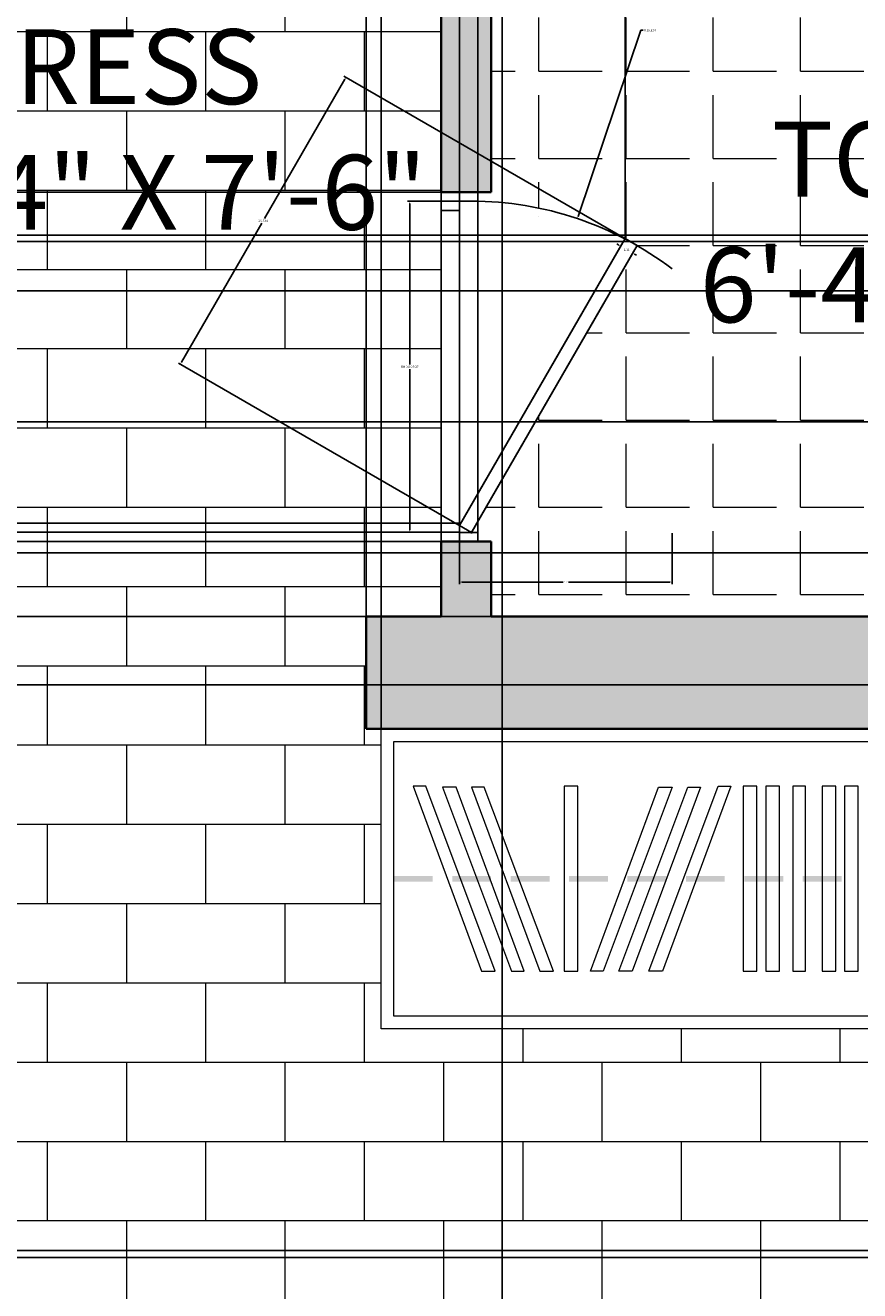
# Model space of a CAD drawing. Units: inches. Extents: x 6 to 575, y 34 to 566.
# Tile 7 of 21: x 84 to 151, y 387 to 488. Entities that reach past the tile are written whole.
import ezdxf

# ---------------------------------------------------------------- set-up
doc = ezdxf.new("R2010")
doc.units = ezdxf.units.IN
for name, color, linetype, lineweight in [('A-ANNO-DIMS', 2, 'Continuous', 18), ('A-AREA-IDEN', 6, 'Continuous', 20), ('A-DOOR-THRS', 8, 'Continuous', 13), ('A-FLOR-CASE', 2, 'Continuous', 18), ('A-FLOR-PATT', 252, 'Continuous', 9), ('A-WALL-PATT', 251, 'Continuous', 9), ('DOORS', 3, 'Continuous', 25), ('WALLS', 7, 'Continuous', 35)]:
    doc.layers.add(name, color=color, linetype=linetype, lineweight=lineweight)
doc.styles.add('PDF Arial Narrow', font='txt')
doc.styles.get("Standard").update_dxf_attribs({"font": 'arial.ttf'})
doc.dimstyles.get("Standard").update_dxf_attribs({"dimtxt": 0.18, "dimasz": 0.18, "dimexe": 0.18, "dimexo": 0.0625, "dimgap": 0.09, "dimtad": 0, "dimtih": 1, "dimtoh": 1, "dimdec": 4, "dimzin": 0, "dimdsep": 46, "dimtxsty": 'Standard', "dimcen": 0.09, "dimadec": 0, "dimazin": 0, "dimtfac": 1, "dimtdec": 4, "dimtofl": 0, "dimtmove": 0, "dimatfit": 3, "dimfxl": 1, "dimtolj": 1, "dimtzin": 0, "dimarcsym": 0})

# ---------------------------------------------------------------- blocks, each defined once
blk = doc.blocks.new('Door - Right Hung 36 in.')
blk.add_lwpolyline([(-0.75, -1.3), (0, 0), (-31.18, 18), (-31.93, 16.7)], close=True)
blk.add_arc((0, 0), 36, 142.6899, 180)
blk = doc.blocks.new('*D17')
at = {"layer": 'A-ANNO-DIMS', "color": 0, "lineweight": -2, "transparency": 16777216}
for p, q in [((119.07, 474.07), (114.97, 474.07)), ((115.15, 473.89), (115.15, 460.99)), ((115.15, 447.72), (115.15, 460.62)), ((119.07, 447.54), (114.97, 447.54))]:
    blk.add_line(p, q, dxfattribs=at)
at = {"layer": 'A-ANNO-DIMS', "color": 0, "transparency": 16777216}
for points in [[(115.12, 473.89), (115.18, 473.89), (115.15, 474.07)], [(115.12, 447.72), (115.18, 447.72), (115.15, 447.54)]]:
    blk.add_solid(points, dxfattribs=at)
at = {"layer": 'Defpoints', "color": 0, "transparency": 16777216}
for p in [(119.13, 474.07), (115.15, 447.54), (119.13, 447.54)]:
    blk.add_point(p, dxfattribs=at)
at = {"layer": 'A-ANNO-DIMS', "color": 0, "transparency": 16777216, "insert": (115.15, 460.8), "char_height": 0.18, "attachment_point": 5}
blk.add_mtext('\\A1;RH DOOR 27', dxfattribs=at)
blk = doc.blocks.new('*D18')
at = {"layer": 'A-ANNO-DIMS', "color": 0, "lineweight": -2, "transparency": 16777216}
for p, q in [((119.13, 447.48), (119.13, 443.38)), ((136.17, 447.48), (136.17, 443.38)), ((119.31, 443.56), (127.44, 443.56)), ((135.99, 443.56), (127.86, 443.56))]:
    blk.add_line(p, q, dxfattribs=at)
at = {"layer": 'A-ANNO-DIMS', "color": 0, "transparency": 16777216}
for points in [[(119.31, 443.59), (119.31, 443.53), (119.13, 443.56)], [(135.99, 443.59), (135.99, 443.53), (136.17, 443.56)]]:
    blk.add_solid(points, dxfattribs=at)
at = {"layer": 'Defpoints', "color": 0, "transparency": 16777216}
for p in [(119.13, 447.54), (136.17, 447.54), (136.17, 443.56)]:
    blk.add_point(p, dxfattribs=at)
at = {"layer": 'A-ANNO-DIMS', "color": 0, "transparency": 16777216, "insert": (127.65, 443.56), "char_height": 0.18, "attachment_point": 5}
blk.add_mtext('\\A1;17', dxfattribs=at)
blk = doc.blocks.new('*D30')
at = {"layer": 'A-ANNO-DIMS', "color": 0, "lineweight": -2, "transparency": 16777216}
for p, q in [((32.6, 539.8), (6.65, 539.8)), ((6.83, 539.62), (6.83, 299.97)), ((6.83, 59.95), (6.83, 299.61)), ((197.62, 59.77), (6.65, 59.77))]:
    blk.add_line(p, q, dxfattribs=at)
at = {"layer": 'A-ANNO-DIMS', "color": 0, "transparency": 16777216}
for points in [[(6.8, 539.62), (6.86, 539.62), (6.83, 539.8)], [(6.8, 59.95), (6.86, 59.95), (6.83, 59.77)]]:
    blk.add_solid(points, dxfattribs=at)
at = {"layer": 'Defpoints', "color": 0, "transparency": 16777216}
for p in [(32.66, 539.8), (6.83, 59.77), (197.69, 59.77)]:
    blk.add_point(p, dxfattribs=at)
at = {"layer": 'A-ANNO-DIMS', "color": 0, "transparency": 16777216, "insert": (6.83, 299.79), "char_height": 0.18, "attachment_point": 5}
blk.add_mtext('\\A1;480', dxfattribs=at)
blk = doc.blocks.new('*D52')
at = {"layer": 'A-ANNO-DIMS', "color": 0, "lineweight": -2, "transparency": 16777216}
for p, q in [((437.62, 471.35), (6.65, 471.35)), ((6.83, 471.17), (6.83, 453.51)), ((6.83, 435.49), (6.83, 453.15)), ((437.62, 435.31), (6.65, 435.31))]:
    blk.add_line(p, q, dxfattribs=at)
at = {"layer": 'A-ANNO-DIMS', "color": 0, "transparency": 16777216}
for points in [[(6.8, 471.17), (6.86, 471.17), (6.83, 471.35)], [(6.8, 435.49), (6.86, 435.49), (6.83, 435.31)]]:
    blk.add_solid(points, dxfattribs=at)
at = {"layer": 'Defpoints', "color": 0, "transparency": 16777216}
for p in [(6.83, 471.35), (437.69, 471.35), (437.69, 435.31)]:
    blk.add_point(p, dxfattribs=at)
at = {"layer": 'A-ANNO-DIMS', "color": 0, "transparency": 16777216, "insert": (6.83, 453.33), "char_height": 0.18, "attachment_point": 5}
blk.add_mtext('\\A1;36.045', dxfattribs=at)
blk = doc.blocks.new('*D55')
at = {"layer": 'A-ANNO-DIMS', "color": 0, "lineweight": -2, "transparency": 16777216}
for p, q in [((41.66, 286.13), (41.66, 565.81)), ((122.56, 286.13), (122.56, 565.81)), ((41.84, 565.63), (81.79, 565.63)), ((122.38, 565.63), (82.44, 565.63))]:
    blk.add_line(p, q, dxfattribs=at)
at = {"layer": 'A-ANNO-DIMS', "color": 0, "transparency": 16777216}
for points in [[(41.84, 565.66), (41.84, 565.6), (41.66, 565.63)], [(122.38, 565.66), (122.38, 565.6), (122.56, 565.63)]]:
    blk.add_solid(points, dxfattribs=at)
at = {"layer": 'Defpoints', "color": 0, "transparency": 16777216}
for p in [(122.56, 565.63), (41.66, 286.06), (122.56, 286.06)]:
    blk.add_point(p, dxfattribs=at)
at = {"layer": 'A-ANNO-DIMS', "color": 0, "transparency": 16777216, "insert": (82.11, 565.63), "char_height": 0.18, "attachment_point": 5}
blk.add_mtext('\\A1;80.9', dxfattribs=at)
blk = doc.blocks.new('*D67')
at = {"layer": 'A-ANNO-DIMS', "color": 0, "lineweight": -2, "transparency": 16777216}
for p, q in [((82.89, 440.86), (82.89, 565.81)), ((111.66, 440.86), (111.66, 565.81)), ((83.07, 565.63), (96.81, 565.63)), ((111.48, 565.63), (97.74, 565.63))]:
    blk.add_line(p, q, dxfattribs=at)
at = {"layer": 'A-ANNO-DIMS', "color": 0, "transparency": 16777216}
for points in [[(83.07, 565.66), (83.07, 565.6), (82.89, 565.63)], [(111.48, 565.66), (111.48, 565.6), (111.66, 565.63)]]:
    blk.add_solid(points, dxfattribs=at)
at = {"layer": 'Defpoints', "color": 0, "transparency": 16777216}
for p in [(111.66, 565.63), (82.89, 440.8), (111.66, 440.8)]:
    blk.add_point(p, dxfattribs=at)
at = {"layer": 'A-ANNO-DIMS', "color": 0, "transparency": 16777216, "insert": (97.28, 565.63), "char_height": 0.18, "attachment_point": 5}
blk.add_mtext('\\A1;28.767', dxfattribs=at)
blk = doc.blocks.new('*D109')
at = {"layer": 'A-ANNO-DIMS', "color": 0, "lineweight": -2, "transparency": 16777216}
for p, q in [((112.85, 431.86), (112.85, 565.81)), ((197.66, 431.86), (197.66, 565.81)), ((113.03, 565.63), (154.93, 565.63)), ((197.48, 565.63), (155.58, 565.63))]:
    blk.add_line(p, q, dxfattribs=at)
at = {"layer": 'A-ANNO-DIMS', "color": 0, "transparency": 16777216}
for points in [[(113.03, 565.66), (113.03, 565.6), (112.85, 565.63)], [(197.48, 565.66), (197.48, 565.6), (197.66, 565.63)]]:
    blk.add_solid(points, dxfattribs=at)
at = {"layer": 'Defpoints', "color": 0, "transparency": 16777216}
for p in [(197.66, 565.63), (112.85, 431.8), (197.66, 431.8)]:
    blk.add_point(p, dxfattribs=at)
at = {"layer": 'A-ANNO-DIMS', "color": 0, "transparency": 16777216, "insert": (155.25, 565.63), "char_height": 0.18, "attachment_point": 5}
blk.add_mtext('\\A1;84.8', dxfattribs=at)
blk = doc.blocks.new('*D132')
at = {"layer": 'A-ANNO-DIMS', "color": 0, "lineweight": -2, "transparency": 16777216}
for p, q in [((288.54, 390), (6.65, 390)), ((6.83, 389.82), (6.83, 366.19)), ((6.83, 342.19), (6.83, 365.82)), ((288.54, 342.01), (6.65, 342.01))]:
    blk.add_line(p, q, dxfattribs=at)
at = {"layer": 'A-ANNO-DIMS', "color": 0, "transparency": 16777216}
for points in [[(6.8, 389.82), (6.86, 389.82), (6.83, 390)], [(6.8, 342.19), (6.86, 342.19), (6.83, 342.01)]]:
    blk.add_solid(points, dxfattribs=at)
at = {"layer": 'Defpoints', "color": 0, "transparency": 16777216}
for p in [(6.83, 390), (288.6, 390), (288.6, 342.01)]:
    blk.add_point(p, dxfattribs=at)
at = {"layer": 'A-ANNO-DIMS', "color": 0, "transparency": 16777216, "insert": (6.83, 366), "char_height": 0.18, "attachment_point": 5}
blk.add_mtext('\\A1;47.98', dxfattribs=at)
blk = doc.blocks.new('*D136')
at = {"layer": 'A-ANNO-DIMS', "color": 0, "lineweight": -2, "transparency": 16777216}
for p, q in [((206.62, 389.45), (6.65, 389.45)), ((6.83, 389.27), (6.83, 350.19)), ((6.83, 310.75), (6.83, 349.83)), ((206.62, 310.57), (6.65, 310.57))]:
    blk.add_line(p, q, dxfattribs=at)
at = {"layer": 'A-ANNO-DIMS', "color": 0, "transparency": 16777216}
for points in [[(6.8, 389.27), (6.86, 389.27), (6.83, 389.45)], [(6.8, 310.75), (6.86, 310.75), (6.83, 310.57)]]:
    blk.add_solid(points, dxfattribs=at)
at = {"layer": 'Defpoints', "color": 0, "transparency": 16777216}
for p in [(6.83, 389.45), (206.68, 389.45), (206.68, 310.57)]:
    blk.add_point(p, dxfattribs=at)
at = {"layer": 'A-ANNO-DIMS', "color": 0, "transparency": 16777216, "insert": (6.83, 350.01), "char_height": 0.18, "attachment_point": 5}
blk.add_mtext('\\A1;78.88', dxfattribs=at)
blk = doc.blocks.new('*D186')
at = {"layer": 'A-ANNO-DIMS', "color": 0, "lineweight": -2, "transparency": 16777216}
for p, q in [((197.6, 470.84), (6.65, 470.84)), ((6.83, 470.66), (6.83, 456)), ((6.83, 440.98), (6.83, 455.64)), ((176.61, 440.8), (6.65, 440.8))]:
    blk.add_line(p, q, dxfattribs=at)
at = {"layer": 'A-ANNO-DIMS', "color": 0, "transparency": 16777216}
for points in [[(6.8, 470.66), (6.86, 470.66), (6.83, 470.84)], [(6.8, 440.98), (6.86, 440.98), (6.83, 440.8)]]:
    blk.add_solid(points, dxfattribs=at)
at = {"layer": 'Defpoints', "color": 0, "transparency": 16777216}
for p in [(6.83, 470.84), (197.66, 470.84), (176.67, 440.8)]:
    blk.add_point(p, dxfattribs=at)
at = {"layer": 'A-ANNO-DIMS', "color": 0, "transparency": 16777216, "insert": (6.83, 455.82), "char_height": 0.18, "attachment_point": 5}
blk.add_mtext('\\A1;30.04', dxfattribs=at)
blk = doc.blocks.new('*D188')
at = {"layer": 'A-ANNO-DIMS', "color": 0, "lineweight": -2, "transparency": 16777216}
for p, q in [((187.14, 466.88), (6.65, 466.88)), ((6.83, 466.7), (6.83, 456.56)), ((6.83, 446.07), (6.83, 456.2)), ((187.02, 445.89), (6.65, 445.89))]:
    blk.add_line(p, q, dxfattribs=at)
at = {"layer": 'A-ANNO-DIMS', "color": 0, "transparency": 16777216}
for points in [[(6.8, 466.7), (6.86, 466.7), (6.83, 466.88)], [(6.8, 446.07), (6.86, 446.07), (6.83, 445.89)]]:
    blk.add_solid(points, dxfattribs=at)
at = {"layer": 'Defpoints', "color": 0, "transparency": 16777216}
for p in [(6.83, 466.88), (187.2, 466.88), (187.08, 445.89)]:
    blk.add_point(p, dxfattribs=at)
at = {"layer": 'A-ANNO-DIMS', "color": 0, "transparency": 16777216, "insert": (6.83, 456.38), "char_height": 0.18, "attachment_point": 5}
blk.add_mtext('\\A1;20.987', dxfattribs=at)
blk = doc.blocks.new('*D189')
at = {"layer": 'A-ANNO-DIMS', "color": 0, "lineweight": -2, "transparency": 16777216}
for p, q in [((187.08, 456.38), (6.65, 456.38)), ((6.83, 456.2), (6.83, 448.77)), ((6.83, 440.98), (6.83, 448.41)), ((197.6, 440.8), (6.65, 440.8))]:
    blk.add_line(p, q, dxfattribs=at)
at = {"layer": 'A-ANNO-DIMS', "color": 0, "transparency": 16777216}
for points in [[(6.8, 456.2), (6.86, 456.2), (6.83, 456.38)], [(6.8, 440.98), (6.86, 440.98), (6.83, 440.8)]]:
    blk.add_solid(points, dxfattribs=at)
at = {"layer": 'Defpoints', "color": 0, "transparency": 16777216}
for p in [(6.83, 456.38), (187.14, 456.38), (197.66, 440.8)]:
    blk.add_point(p, dxfattribs=at)
at = {"layer": 'A-ANNO-DIMS', "color": 0, "transparency": 16777216, "insert": (6.83, 448.59), "char_height": 0.18, "attachment_point": 5}
blk.add_mtext('\\A1;15.582', dxfattribs=at)
blk = doc.blocks.new('*D197')
at = {"layer": 'A-ANNO-DIMS', "color": 0, "lineweight": -2, "transparency": 16777216}
for p, q in [((117.6, 446.8), (6.65, 446.8)), ((6.83, 446.62), (6.83, 443.98)), ((6.83, 440.98), (6.83, 443.62)), ((117.6, 440.8), (6.65, 440.8))]:
    blk.add_line(p, q, dxfattribs=at)
at = {"layer": 'A-ANNO-DIMS', "color": 0, "transparency": 16777216}
for points in [[(6.8, 446.62), (6.86, 446.62), (6.83, 446.8)], [(6.8, 440.98), (6.86, 440.98), (6.83, 440.8)]]:
    blk.add_solid(points, dxfattribs=at)
at = {"layer": 'Defpoints', "color": 0, "transparency": 16777216}
for p in [(6.83, 446.8), (117.66, 446.8), (117.66, 440.8)]:
    blk.add_point(p, dxfattribs=at)
at = {"layer": 'A-ANNO-DIMS', "color": 0, "transparency": 16777216, "insert": (6.83, 443.8), "char_height": 0.18, "attachment_point": 5}
blk.add_mtext('\\A1;6', dxfattribs=at)
blk = doc.blocks.new('*D198')
at = {"layer": 'A-ANNO-DIMS', "color": 0, "lineweight": -2, "transparency": 16777216}
for p, q in [((117.6, 474.8), (6.65, 474.8)), ((6.83, 474.62), (6.83, 460.98)), ((6.83, 446.98), (6.83, 460.62)), ((117.6, 446.8), (6.65, 446.8))]:
    blk.add_line(p, q, dxfattribs=at)
at = {"layer": 'A-ANNO-DIMS', "color": 0, "transparency": 16777216}
for points in [[(6.8, 474.62), (6.86, 474.62), (6.83, 474.8)], [(6.8, 446.98), (6.86, 446.98), (6.83, 446.8)]]:
    blk.add_solid(points, dxfattribs=at)
at = {"layer": 'Defpoints', "color": 0, "transparency": 16777216}
for p in [(6.83, 474.8), (117.66, 474.8), (117.66, 446.8)]:
    blk.add_point(p, dxfattribs=at)
at = {"layer": 'A-ANNO-DIMS', "color": 0, "transparency": 16777216, "insert": (6.83, 460.8), "char_height": 0.18, "attachment_point": 5}
blk.add_mtext('\\A1;28', dxfattribs=at)
blk = doc.blocks.new('*D199')
at = {"layer": 'A-ANNO-DIMS', "color": 0, "lineweight": -2, "transparency": 16777216}
for p, q in [((109.94, 483.83), (103.5, 472.68)), ((132.35, 471.1), (109.87, 484.07)), ((96.85, 461.16), (103.29, 472.31)), ((119.08, 448.12), (96.61, 461.1))]:
    blk.add_line(p, q, dxfattribs=at)
at = {"layer": 'A-ANNO-DIMS', "color": 0, "transparency": 16777216}
for points in [[(109.91, 483.84), (109.97, 483.81), (110.03, 483.98)], [(96.83, 461.18), (96.88, 461.15), (96.76, 461.01)]]:
    blk.add_solid(points, dxfattribs=at)
at = {"layer": 'Defpoints', "color": 0, "transparency": 16777216}
for p in [(110.03, 483.98), (132.4, 471.07), (119.13, 448.09)]:
    blk.add_point(p, dxfattribs=at)
at = {"layer": 'A-ANNO-DIMS', "color": 0, "transparency": 16777216, "insert": (103.4, 472.5), "char_height": 0.18, "attachment_point": 5}
blk.add_mtext('\\A1;26.534', dxfattribs=at)
blk = doc.blocks.new('*D200')
at = {"layer": 'A-ANNO-DIMS', "color": 0, "lineweight": -2, "transparency": 16777216}
for p, q in [((119.13, 448.15), (119.13, 565.81)), ((132.4, 471.13), (132.4, 565.81)), ((119.31, 565.63), (125.31, 565.63)), ((132.22, 565.63), (126.22, 565.63))]:
    blk.add_line(p, q, dxfattribs=at)
at = {"layer": 'A-ANNO-DIMS', "color": 0, "transparency": 16777216}
for points in [[(119.31, 565.66), (119.31, 565.6), (119.13, 565.63)], [(132.22, 565.66), (132.22, 565.6), (132.4, 565.63)]]:
    blk.add_solid(points, dxfattribs=at)
at = {"layer": 'Defpoints', "color": 0, "transparency": 16777216}
for p in [(132.4, 565.63), (132.4, 471.07), (119.13, 448.09)]:
    blk.add_point(p, dxfattribs=at)
at = {"layer": 'A-ANNO-DIMS', "color": 0, "transparency": 16777216, "insert": (125.77, 565.63), "char_height": 0.18, "attachment_point": 5}
blk.add_mtext('\\A1;13.267', dxfattribs=at)
blk = doc.blocks.new('*D201')
at = {"layer": 'A-ANNO-DIMS', "color": 0, "lineweight": -2, "transparency": 16777216}
for p, q in [((119.16, 448.14), (132.14, 470.62)), ((131.89, 470.55), (131.74, 470.64)), ((120.12, 447.59), (133.1, 470.06)), ((133.16, 469.82), (133.32, 469.73))]:
    blk.add_line(p, q, dxfattribs=at)
at = {"layer": 'A-ANNO-DIMS', "color": 0, "transparency": 16777216}
for points in [[(131.91, 470.58), (131.88, 470.52), (132.05, 470.46)], [(133.18, 469.84), (133.15, 469.79), (133.01, 469.91)]]:
    blk.add_solid(points, dxfattribs=at)
at = {"layer": 'Defpoints', "color": 0, "transparency": 16777216}
for p in [(133.01, 469.91), (119.13, 448.09), (120.09, 447.54)]:
    blk.add_point(p, dxfattribs=at)
at = {"layer": 'A-ANNO-DIMS', "color": 0, "transparency": 16777216, "insert": (132.53, 470.18), "char_height": 0.18, "attachment_point": 5}
blk.add_mtext('\\A1;1.11', dxfattribs=at)
blk = doc.blocks.new('*D202')
at = {"layer": 'A-ANNO-DIMS', "color": 0, "lineweight": -2, "transparency": 16777216}
for p, q in [((117.66, 446.86), (117.66, 565.81)), ((120.61, 446.86), (120.61, 565.81)), ((117.84, 565.63), (118.74, 565.63)), ((120.43, 565.63), (119.53, 565.63))]:
    blk.add_line(p, q, dxfattribs=at)
at = {"layer": 'A-ANNO-DIMS', "color": 0, "transparency": 16777216}
for points in [[(117.84, 565.66), (117.84, 565.6), (117.66, 565.63)], [(120.43, 565.66), (120.43, 565.6), (120.61, 565.63)]]:
    blk.add_solid(points, dxfattribs=at)
at = {"layer": 'Defpoints', "color": 0, "transparency": 16777216}
for p in [(120.61, 565.63), (117.66, 446.8), (120.61, 446.8)]:
    blk.add_point(p, dxfattribs=at)
at = {"layer": 'A-ANNO-DIMS', "color": 0, "transparency": 16777216, "insert": (119.13, 565.63), "char_height": 0.18, "attachment_point": 5}
blk.add_mtext('\\A1;2.948', dxfattribs=at)
blk = doc.blocks.new('*D203')
at = {"layer": 'A-ANNO-DIMS', "color": 0, "lineweight": -2, "transparency": 16777216}
for p, q in [((117.6, 448.28), (6.65, 448.28)), ((6.83, 448.1), (6.83, 447.72)), ((6.83, 446.98), (6.83, 447.36)), ((117.6, 446.8), (6.65, 446.8))]:
    blk.add_line(p, q, dxfattribs=at)
at = {"layer": 'A-ANNO-DIMS', "color": 0, "transparency": 16777216}
for points in [[(6.8, 448.1), (6.86, 448.1), (6.83, 448.28)], [(6.8, 446.98), (6.86, 446.98), (6.83, 446.8)]]:
    blk.add_solid(points, dxfattribs=at)
at = {"layer": 'Defpoints', "color": 0, "transparency": 16777216}
for p in [(6.83, 448.28), (117.66, 448.28), (117.66, 446.8)]:
    blk.add_point(p, dxfattribs=at)
at = {"layer": 'A-ANNO-DIMS', "color": 0, "transparency": 16777216, "insert": (6.83, 447.54), "char_height": 0.18, "attachment_point": 5}
blk.add_mtext('\\A1;1.474', dxfattribs=at)
blk = doc.blocks.new('*D204')
at = {"layer": 'A-ANNO-DIMS', "color": 0, "lineweight": -2, "transparency": 16777216}
for p, q in [((119.07, 448.28), (6.65, 448.28)), ((6.83, 448.1), (6.83, 447.72)), ((119.07, 447.54), (6.65, 447.54)), ((6.83, 447.36), (6.65, 447.36)), ((6.83, 447.54), (6.83, 447.36))]:
    blk.add_line(p, q, dxfattribs=at)
at = {"layer": 'A-ANNO-DIMS', "color": 0, "transparency": 16777216}
for points in [[(6.8, 448.1), (6.86, 448.1), (6.83, 448.28)], [(6.8, 447.72), (6.86, 447.72), (6.83, 447.54)]]:
    blk.add_solid(points, dxfattribs=at)
at = {"layer": 'Defpoints', "color": 0, "transparency": 16777216}
for p in [(119.13, 448.28), (6.83, 447.54), (119.13, 447.54)]:
    blk.add_point(p, dxfattribs=at)
at = {"layer": 'A-ANNO-DIMS', "color": 0, "transparency": 16777216, "insert": (6.25, 447.36), "char_height": 0.18, "attachment_point": 5}
blk.add_mtext('\\A1;0.737', dxfattribs=at)
blk = doc.blocks.new('*D205')
at = {"layer": 'A-ANNO-DIMS', "color": 0, "lineweight": -2, "transparency": 16777216}
for p, q in [((119.13, 447.6), (119.13, 565.81)), ((120.61, 447.6), (120.61, 565.81)), ((119.31, 565.63), (119.48, 565.63)), ((120.43, 565.63), (120.25, 565.63))]:
    blk.add_line(p, q, dxfattribs=at)
at = {"layer": 'A-ANNO-DIMS', "color": 0, "transparency": 16777216}
for points in [[(119.31, 565.66), (119.31, 565.6), (119.13, 565.63)], [(120.43, 565.66), (120.43, 565.6), (120.61, 565.63)]]:
    blk.add_solid(points, dxfattribs=at)
at = {"layer": 'Defpoints', "color": 0, "transparency": 16777216}
for p in [(120.61, 565.63), (119.13, 447.54), (120.61, 447.54)]:
    blk.add_point(p, dxfattribs=at)
at = {"layer": 'A-ANNO-DIMS', "color": 0, "transparency": 16777216, "insert": (119.87, 565.63), "char_height": 0.18, "attachment_point": 5}
blk.add_mtext('\\A1;1.474', dxfattribs=at)
blk = doc.blocks.new('*D229')
at = {"layer": 'A-ANNO-DIMS', "color": 0, "lineweight": -2, "transparency": 16777216}
for p, q in [((133.67, 487.76), (128.63, 472.85)), ((133.85, 487.76), (133.67, 487.76)), ((120, 447.54), (120.18, 447.54)), ((120.09, 447.45), (120.09, 447.63))]:
    blk.add_line(p, q, dxfattribs=at)
at = {"layer": 'A-ANNO-DIMS', "color": 0, "transparency": 16777216}
blk.add_solid([(128.61, 472.86), (128.66, 472.84), (128.58, 472.68)], dxfattribs=at)
at = {"layer": 'Defpoints', "color": 0, "transparency": 16777216}
for p in [(128.58, 472.68), (120.09, 447.54)]:
    blk.add_point(p, dxfattribs=at)
at = {"layer": 'A-ANNO-DIMS', "color": 0, "transparency": 16777216, "insert": (134.4, 487.76), "char_height": 0.18, "attachment_point": 5}
blk.add_mtext('\\A1;R26.534', dxfattribs=at)

msp = doc.modelspace()

# ---------------------------------------------------------------- hatches: boundary and pattern name
at = {"layer": 'A-FLOR-PATT'}
h = msp.add_hatch(dxfattribs=at)
h.set_pattern_fill('ANGLE', color=256)
h.set_pattern_definition([(0, (-98.035, 170.1465), (0, 6.985), [5.08, -1.905]), (90, (-98.035, 170.1465), (-6.985, 4e-16), [5.08, -1.905])])
edge = h.paths.add_edge_path()
edge.add_line((191.6511, 494.1664), (190.4028, 493.9036))
edge.add_line((190.4028, 493.9036), (189.6226, 493.6983))
edge.add_line((189.6226, 493.6983), (188.2183, 493.3862))
edge.add_line((188.2183, 493.3862), (187.2685, 493.2437))
edge.add_line((187.2685, 493.2437), (187.204, 493.2302))
edge.add_line((187.204, 493.2302), (187.0709, 493.2141))
edge.add_line((187.0709, 493.2141), (185.0975, 492.9181))
edge.add_line((185.0975, 492.9181), (185.0904, 492.9751))
edge.add_line((185.0904, 492.9751), (183.6001, 492.7952))
edge.add_line((183.6001, 492.7952), (183.5371, 492.7621))
edge.add_line((183.5371, 492.7621), (181.5041, 492.4232))
edge.add_spline(control_points=[(181.5178, 492.4356), (181.2536, 492.4138), (180.9898, 492.4), (180.727, 492.3941)], knot_values=[2.92921633, 2.92921633, 2.92921633, 2.92921633, 3, 3, 3, 3], degree=3, periodic=0)
edge.add_line((180.727, 492.3941), (180.4943, 492.372))
edge.add_line((180.4943, 492.372), (180.175, 492.3932))
edge.add_spline(control_points=[(180.175, 492.3932), (179.0187, 492.4156), (177.8901, 492.5895), (176.8377, 492.8977)], knot_values=[2.56593531, 2.56593531, 2.56593531, 2.56593531, 2.87949124, 2.87949124, 2.87949124, 2.87949124], degree=3, periodic=0)
edge.add_line((176.8377, 492.8977), (176.5264, 492.9696))
edge.add_spline(control_points=[(176.656, 492.9525), (176.2658, 493.0735), (175.8866, 493.2132), (175.521, 493.3707)], knot_values=[2.43053183, 2.43053183, 2.43053183, 2.43053183, 2.54781219, 2.54781219, 2.54781219, 2.54781219], degree=3, periodic=0)
edge.add_line((175.521, 493.3707), (175.267, 493.4642))
edge.add_line((175.267, 493.4642), (175.098, 493.5637))
edge.add_spline(control_points=[(175.098, 493.5637), (173.9351, 494.1251), (172.9292, 494.8734), (172.1696, 495.7766)], knot_values=[2, 2, 2, 2, 2.38461715, 2.38461715, 2.38461715, 2.38461715], degree=3, periodic=0)
edge.add_line((172.9656, 494.9581), (172.8363, 495.1004))
edge.add_spline(control_points=[(175.098, 493.5637), (173.9351, 494.1251), (172.9292, 494.8734), (172.1696, 495.7766)], knot_values=[2, 2, 2, 2, 2.38461715, 2.38461715, 2.38461715, 2.38461715], degree=3, periodic=0)
edge.add_line((171.9925, 495.9563), (171.8762, 496.1888))
edge.add_spline(control_points=[(172.1696, 495.7766), (170.1947, 498.1251), (170.2393, 501.0999), (172.2842, 503.4158)], knot_values=[1, 1, 1, 1, 2, 2, 2, 2], degree=3, periodic=0)
edge.add_line((170.6556, 499.1388), (170.6881, 499.323))
edge.add_spline(control_points=[(172.1696, 495.7766), (170.1947, 498.1251), (170.2393, 501.0999), (172.2842, 503.4158)], knot_values=[1, 1, 1, 1, 2, 2, 2, 2], degree=3, periodic=0)
edge.add_spline(control_points=[(172.2842, 503.4158), (174.3291, 505.7317), (178.0076, 506.9734), (181.7304, 506.6045)], knot_values=[0, 0, 0, 0, 1, 1, 1, 1], degree=3, periodic=0)
edge.add_line((174.0548, 504.9343), (174.2554, 505.022))
edge.add_spline(control_points=[(172.2842, 503.4158), (174.3291, 505.7317), (178.0076, 506.9734), (181.7304, 506.6045)], knot_values=[0, 0, 0, 0, 1, 1, 1, 1], degree=3, periodic=0)
edge.add_line((178.4031, 506.5313), (178.1947, 506.4718))
edge.add_spline(control_points=[(172.2842, 503.4158), (174.3291, 505.7317), (178.0076, 506.9734), (181.7304, 506.6045)], knot_values=[0, 0, 0, 0, 1, 1, 1, 1], degree=3, periodic=0)
edge.add_line((181.5796, 506.6123), (181.6459, 506.5957))
edge.add_arc((179.34, 495.0824), 11.742, 73.636084, 78.674278, ccw=False)
edge.add_arc((178.5598, 454.8227), 51.688, 83.52982, 85.463383, ccw=False)
edge.add_line((184.3843, 506.1814), (184.5513, 506.1814))
edge.add_line((184.5513, 506.1814), (184.7887, 506.134))
edge.add_arc((178.5598, 454.8227), 51.688, 75.328548, 83.07845, ccw=False)
edge.add_line((191.6511, 504.8253), (191.6511, 530.801))
edge.add_line((191.6511, 530.801), (184.6586, 530.801))
edge.add_line((184.6586, 530.801), (160.6586, 530.801))
edge.add_line((160.6586, 530.801), (157.8686, 530.801))
edge.add_line((157.8686, 530.801), (157.8686, 488.7831))
edge.add_line((157.8686, 488.7831), (121.6586, 488.7831))
edge.add_line((121.6586, 488.7831), (121.6586, 474.801))
edge.add_line((121.6586, 474.801), (120.6068, 474.801))
edge.add_line((120.6068, 474.801), (120.6068, 474.0666))
edge.add_arc((120.0902, 447.538), 26.5336, 62.388015, 88.884314, ccw=False)
edge.add_line((132.388, 471.0496), (132.3995, 471.0696))
edge.add_line((132.3995, 471.0696), (133.357, 470.5168))
edge.add_line((133.357, 470.5168), (120.0902, 447.538))
edge.add_line((120.0902, 447.538), (120.6068, 447.538))
edge.add_line((120.6068, 447.538), (121.6586, 446.801))
edge.add_line((121.6586, 446.801), (121.6586, 440.801))
edge.add_line((121.6586, 440.801), (176.6714, 440.801))
edge.add_line((176.6714, 440.801), (176.6714, 470.8385))
edge.add_line((176.6714, 470.8385), (191.6511, 470.8385))
edge.add_line((191.6511, 470.8385), (191.6511, 494.1664))
h = msp.add_hatch(dxfattribs=at)
h.set_pattern_fill('BRICK', color=256)
h.set_pattern_definition([(0, (-98.035, 170.1465), (0, 6.35), []), (90, (-98.035, 170.147), (-12.7, 8e-16), [6.35, -6.35]), (90, (-91.685, 170.147), (-12.7, 8e-16), [-6.35, 6.35])])
h.paths.add_polyline_path([(180.8711, 269.7588), (182.4439, 270.6668), (182.4628, 270.6341, -0.11619827), (201.8275, 275.5902), (201.8275, 276.801), (197.6586, 276.801), (197.6586, 293.1641), (182.6401, 293.1641), (182.6401, 348.324), (197.6586, 348.324), (197.6586, 407.7709), (112.8513, 407.7709), (112.8513, 431.801), (111.6586, 431.801), (111.6586, 440.801), (117.6586, 440.801), (117.6586, 446.801), (117.6586, 448.2751), (117.6586, 473.3269), (117.6586, 474.801), (117.6586, 515.5941), (100.2533, 515.5941, -1), (83.0548, 515.5941), (65.6494, 515.5941), (65.6494, 440.801), (82.8918, 440.801), (82.8918, 431.801), (82.8918, 407.7709), (41.6586, 407.7709), (41.6586, 379.0637), (62.6459, 379.0637), (62.6459, 358.0764), (122.565, 358.0764), (122.565, 286.0643), (62.6459, 286.0643), (62.6459, 265.077), (41.6586, 265.077), (41.6586, 224.801), (41.6586, 212.801), (71.6586, 212.801), (167.6586, 212.801), (197.6586, 212.801), (197.6586, 230.801), (201.8157, 230.801), (201.8157, 233.4817)])
h.paths.add_polyline_path([(133.3414, 245.1275), (133.3317, 245.1352), (133.3317, 245.104)], flags=16)
h.paths.add_polyline_path([(133.3317, 222.1662), (85.3496, 222.1662), (85.3496, 243.7443, -0.50090726), (87.1831, 246.1963), (107.4292, 246.1963), (111.2522, 246.1963), (131.4202, 246.1963, -0.41421356), (133.3317, 244.2848)], flags=16)
h.paths.add_polyline_path([(72.7105, 244.4018), (72.7105, 220.3718), (48.6804, 220.3718), (48.6804, 244.4018)], flags=16)
h.paths.add_polyline_path([(71.7466, 237.8955, -1), (59.8096, 237.8955, -1)], flags=0)
at = {"layer": 'A-WALL-PATT'}
h = msp.add_hatch(color=256, dxfattribs=at)
h.dxf.hatch_style = 1
h.paths.add_polyline_path([(160.6586, 539.801), (32.6586, 539.801), (32.6586, 272.801), (41.6586, 272.801), (41.6586, 286.0643), (41.6586, 358.0764), (41.6586, 379.0637), (41.6586, 407.7709), (41.6194, 407.7709), (41.6194, 431.801), (82.8918, 431.801), (82.8918, 440.801), (65.6494, 440.801), (65.6494, 440.7732), (41.6194, 440.7732), (41.6194, 515.5941), (41.6586, 530.801), (117.6586, 530.801), (117.6586, 474.801), (120.6068, 474.801), (121.6586, 474.801), (121.6586, 530.801), (137.4275, 530.801), (137.4275, 530.8356), (141.2505, 530.8356), (160.6586, 530.801)])
h.paths.add_polyline_path([(71.6586, 212.801), (41.6586, 212.801), (41.6586, 224.801), (32.6586, 224.801), (32.6586, 203.801), (71.6586, 203.801)])
h.paths.add_polyline_path([(206.6586, 215.801), (246.6586, 215.801), (246.6586, 224.801), (206.6586, 224.801), (206.6586, 230.801), (201.8157, 230.801), (197.6586, 230.801), (197.6586, 212.801), (167.6586, 212.801), (167.6586, 203.801), (206.6586, 203.801)])
h.paths.add_polyline_path([(383.6586, 224.801), (334.6586, 224.801), (334.6586, 215.801), (374.6586, 215.801), (374.6586, 203.801), (384.0753, 203.801), (407.6586, 203.801), (407.6586, 212.801), (383.6586, 212.801)])
h.paths.add_polyline_path([(548.6586, 270.801), (539.6586, 270.801), (539.6586, 212.801), (515.6586, 212.801), (515.6586, 203.801), (548.6586, 203.801)])
h.paths.add_polyline_path([(548.6586, 412.801), (545.7108, 412.801), (539.6586, 412.801), (539.6586, 382.801), (433.708, 382.801), (433.708, 378.801), (539.6586, 378.801), (539.6586, 366.801), (548.6586, 366.801)])
h.paths.add_polyline_path([(548.6586, 539.801), (455.9436, 539.801), (455.9436, 530.801), (539.6586, 530.801), (539.6586, 440.801), (548.6586, 440.801)])
h.paths.add_polyline_path([(407.9436, 539.801), (362.6586, 539.801), (362.6586, 530.801), (374.6586, 530.801), (374.6586, 452.801), (354.6586, 452.801), (354.6586, 448.801), (374.6586, 448.801), (374.6586, 278.801), (383.6586, 278.801), (383.6586, 530.801), (407.9436, 530.801)])
h.paths.add_polyline_path([(338.6586, 539.801), (320.6586, 539.801), (320.6586, 530.801), (322.6586, 530.801), (322.6586, 448.801), (326.6586, 448.801), (326.6586, 530.801), (338.6586, 530.801)])
h.paths.add_polyline_path([(272.6586, 539.801), (184.6586, 539.801), (184.6586, 530.801), (197.6586, 530.801), (197.6586, 440.801), (176.6714, 440.801), (121.6586, 440.801), (121.6586, 446.801), (117.6586, 446.801), (117.6586, 440.801), (111.6586, 440.801), (111.6586, 431.801), (197.6586, 431.801), (197.6586, 407.7709), (197.6586, 276.801), (206.6586, 276.801), (206.6586, 530.801), (272.6586, 530.801)])

# ---------------------------------------------------------------- linework, layer by layer
at = {"layer": 'A-DOOR-THRS'}
msp.add_line((117.6586, 473.3269), (117.6586, 448.2751), dxfattribs=at)
at = {"layer": 'A-FLOR-CASE'}
for points in [[(197.6586, 407.7709), (112.8513, 407.7709), (112.8513, 431.801), (197.6586, 431.801)], [(196.6444, 408.7852), (113.8656, 408.7852), (113.8656, 430.7867), (196.6444, 430.7867)], [(121.9796, 412.3741), (116.4402, 427.1978), (115.426, 427.1978), (120.8873, 412.3741)], [(124.3202, 412.3741), (118.8588, 427.1198), (117.7665, 427.1198), (123.3059, 412.3741)], [(126.6608, 412.3741), (121.1214, 427.1198), (120.1071, 427.1198), (125.5685, 412.3741)], [(128.6113, 412.3741), (128.6113, 427.1978), (127.519, 427.1978), (127.519, 412.3741)], [(129.6255, 412.3741), (135.0869, 427.1198), (136.1792, 427.1198), (130.6398, 412.3741)], [(131.8881, 412.3741), (137.4275, 427.1198), (138.4417, 427.1198), (132.9804, 412.3741)], [(134.3067, 412.3741), (139.8461, 427.1978), (140.8604, 427.1978), (135.399, 412.3741)], [(142.9669, 412.3741), (142.9669, 427.1978), (141.8746, 427.1978), (141.8746, 412.3741)], [(144.7613, 412.3741), (144.7613, 427.1978), (143.6691, 427.1978), (143.6691, 412.3741)], [(146.8679, 412.3741), (146.8679, 427.1978), (145.8536, 427.1978), (145.8536, 412.3741)], [(149.2865, 412.3741), (149.2865, 427.1978), (148.1942, 427.1978), (148.1942, 412.3741)], [(151.0809, 412.3741), (151.0809, 427.1978), (149.9887, 427.1978), (149.9887, 412.3741)]]:
    msp.add_lwpolyline(points, close=True, dxfattribs=at)
at = {"layer": 'A-FLOR-CASE', "transparency": 33554559}
for points in [[(113.8656, 420.02), (113.8656, 419.5519), (116.9864, 420.02)], [(113.8656, 419.5519), (116.9864, 420.02), (116.9864, 419.5519)], [(118.5467, 420.02), (118.5467, 419.5519), (121.6675, 420.02)], [(118.5467, 419.5519), (121.6675, 420.02), (121.6675, 419.5519)], [(123.2279, 420.02), (123.2279, 419.5519), (126.3487, 420.02)], [(123.2279, 419.5519), (126.3487, 420.02), (126.3487, 419.5519)], [(127.9091, 420.02), (127.9091, 419.5519), (131.0299, 420.02)], [(127.9091, 419.5519), (131.0299, 420.02), (131.0299, 419.5519)], [(132.5903, 420.02), (132.5903, 419.5519), (135.7111, 420.02)], [(132.5903, 419.5519), (135.7111, 420.02), (135.7111, 419.5519)], [(137.2715, 420.02), (137.2715, 419.5519), (140.3922, 420.02)], [(137.2715, 419.5519), (140.3922, 420.02), (140.3922, 419.5519)], [(141.9526, 420.02), (141.9526, 419.5519), (145.0734, 420.02)], [(141.9526, 419.5519), (145.0734, 420.02), (145.0734, 419.5519)], [(146.6338, 420.02), (146.6338, 419.5519), (149.7546, 420.02)], [(146.6338, 419.5519), (149.7546, 420.02), (149.7546, 419.5519)]]:
    msp.add_solid(points, dxfattribs=at)
at = {"layer": 'DOORS'}
for points in [[(117.6586, 473.3269), (117.6586, 474.801), (120.6068, 474.801), (120.6068, 474.0639), (119.1327, 474.0639), (119.1327, 473.3269)], [(117.6586, 448.2751), (117.6586, 446.801), (120.6068, 446.801), (120.6068, 447.538), (119.1327, 447.538), (119.1327, 448.2751)]]:
    msp.add_lwpolyline(points, close=True, dxfattribs=at)
at = {"layer": 'WALLS'}
for p, q in [((117.6586, 530.801), (117.6586, 474.801)), ((121.6586, 530.801), (121.6586, 474.801)), ((121.6586, 474.801), (117.6586, 474.801)), ((121.6586, 446.801), (117.6586, 446.801)), ((117.6586, 446.801), (117.6586, 440.801)), ((121.6586, 440.801), (121.6586, 446.801)), ((121.6586, 446.801), (121.6586, 440.801)), ((111.6586, 440.801), (111.6586, 431.801)), ((111.6586, 440.801), (117.6586, 440.801)), ((121.6586, 440.801), (197.6586, 440.801)), ((111.6586, 431.801), (197.6586, 431.801))]:
    msp.add_line(p, q, dxfattribs=at)

# ---------------------------------------------------------------- block references
at = {"layer": 'DOORS', "xscale": 0.7370445650527652, "yscale": 0.7370445650527652, "zscale": 0.7370445650527652, "rotation": 270}
msp.add_blockref('Door - Right Hung 36 in.', (120.0902, 447.538), dxfattribs=at)

# ---------------------------------------------------------------- texts
at = {"layer": 'A-AREA-IDEN', "attachment_point": 4, "style": 'PDF Arial Narrow'}
for s, insert, char_height in [('DRESS', (77.9064, 484.0646), 6.0005), ('TOILET', (144.1573, 476.6524), 6.0005), ('6\'-4" X 7\'-6"', (71.9766, 473.9997), 6.000503), ('6\'-4" X 7\'-6"', (138.3837, 466.5875), 6.000503)]:
    msp.add_mtext(s, dxfattribs=dict(at, insert=insert, char_height=char_height))

# ---------------------------------------------------------------- dimensions: what is measured, and where the dimension line sits
at = {"layer": 'A-ANNO-DIMS'}
for base, p1, p2, override, picture, middle in [((122.565, 565.631), (41.6586, 286.0643), (122.565, 286.0643), {"dimdec": 1, "dimlfac": 1, "dimrnd": 0, "dimzin": 0, "dimdsep": 46, "dimlunit": 2}, '*D55', (82.1118, 565.631)), ((111.6586, 565.631), (82.8918, 440.801), (111.6586, 440.801), {"dimdec": 3, "dimlfac": 1, "dimrnd": 0, "dimzin": 0, "dimdsep": 46, "dimlunit": 2}, '*D67', (97.2752, 565.631)), ((197.6586, 565.631), (112.8513, 431.801), (197.6586, 431.801), {"dimdec": 1, "dimlfac": 1, "dimrnd": 0, "dimzin": 0, "dimdsep": 46, "dimlunit": 2}, '*D109', (155.255, 565.631)), ((120.6068, 565.631), (117.6586, 446.801), (120.6068, 446.801), {"dimdec": 3, "dimlfac": 1, "dimrnd": 0, "dimzin": 0, "dimdsep": 46, "dimlunit": 2}, '*D202', (119.1327, 565.631)), ((132.3995, 565.631), (119.1327, 448.0908), (132.3995, 471.0696), {"dimdec": 3, "dimlfac": 1, "dimrnd": 0, "dimzin": 0, "dimdsep": 46, "dimlunit": 2}, '*D200', (125.7661, 565.631)), ((120.6068, 565.631), (119.1327, 447.538), (120.6068, 447.538), {"dimdec": 3, "dimlfac": 1, "dimrnd": 0, "dimzin": 0, "dimdsep": 46, "dimlunit": 2}, '*D205', (119.8698, 565.631)), ((136.173, 443.558), (119.1327, 447.538), (136.173, 447.538), {"dimdec": 0, "dimlfac": 1, "dimrnd": 0, "dimzin": 0, "dimdsep": 46, "dimlunit": 2}, '*D18', (127.6529, 443.558))]:
    dim = msp.add_linear_dim(base=base, p1=p1, p2=p2, dimstyle='Standard', override=override, dxfattribs=at)
    dim.commit()
    dim.dimension.update_dxf_attribs({"geometry": picture, "text_midpoint": middle})
for base, p1, p2, angle, override, picture, middle in [((6.8286, 59.7747), (32.6586, 539.801), (197.6872, 59.7747), 90, {"dimdec": 0, "dimlfac": 1, "dimrnd": 0, "dimzin": 0, "dimdsep": 46, "dimlunit": 2}, '*D30', (6.8286, 299.7878)), ((110.0301, 483.9846), (119.1327, 448.0908), (132.3995, 471.0696), 60, {"dimdec": 3, "dimlfac": 1, "dimrnd": 0, "dimzin": 0, "dimdsep": 46, "dimlunit": 2}, '*D199', (103.3967, 472.4952)), ((6.8286, 474.801), (117.6586, 446.801), (117.6586, 474.801), 90, {"dimdec": 0, "dimlfac": 1, "dimrnd": 0, "dimzin": 0, "dimdsep": 46, "dimlunit": 2}, '*D198', (6.8286, 460.801)), ((6.8286, 471.3533), (437.687, 435.3082), (437.687, 471.3533), 90, {"dimdec": 3, "dimlfac": 1, "dimrnd": 0, "dimzin": 0, "dimdsep": 46, "dimlunit": 2}, '*D52', (6.8286, 453.3307)), ((6.8286, 470.8385), (176.6714, 440.801), (197.6586, 470.8385), 90, {"dimdec": 2, "dimlfac": 1, "dimrnd": 0, "dimzin": 0, "dimdsep": 46, "dimlunit": 2}, '*D186', (6.8286, 455.8198)), ((133.0052, 469.9075), (119.1327, 448.0908), (120.0902, 447.538), 330, {"dimdec": 2, "dimlfac": 1, "dimrnd": 0, "dimzin": 0, "dimdsep": 46, "dimlunit": 2}, '*D201', (132.5265, 470.1839)), ((6.8286, 466.8767), (187.0809, 445.8894), (187.2036, 466.8767), 90, {"dimdec": 3, "dimlfac": 1, "dimrnd": 0, "dimzin": 0, "dimdsep": 46, "dimlunit": 2}, '*D188', (6.8286, 456.3831)), ((6.8286, 456.3831), (197.6586, 440.801), (187.1423, 456.3831), 90, {"dimdec": 3, "dimlfac": 1, "dimrnd": 0, "dimzin": 0, "dimdsep": 46, "dimlunit": 2}, '*D189', (6.8286, 448.592)), ((6.8286, 447.538), (119.1327, 448.2751), (119.1327, 447.538), 90, {"dimdec": 3, "dimlfac": 1, "dimrnd": 0, "dimzin": 0, "dimdsep": 46, "dimlunit": 2}, '*D204', (6.2549, 447.358)), ((6.8286, 448.2751), (117.6586, 446.801), (117.6586, 448.2751), 90, {"dimdec": 3, "dimlfac": 1, "dimrnd": 0, "dimzin": 0, "dimdsep": 46, "dimlunit": 2}, '*D203', (6.8286, 447.538)), ((6.8286, 446.801), (117.6586, 440.801), (117.6586, 446.801), 90, {"dimdec": 0, "dimlfac": 1, "dimrnd": 0, "dimzin": 0, "dimdsep": 46, "dimlunit": 2}, '*D197', (6.8286, 443.801)), ((6.8286, 389.9952), (288.603, 342.0131), (288.603, 389.9952), 90, {"dimdec": 2, "dimlfac": 1, "dimrnd": 0, "dimzin": 0, "dimdsep": 46, "dimlunit": 2}, '*D132', (6.8286, 366.0042)), ((6.8286, 389.449), (206.6824, 310.5712), (206.6824, 389.449), 90, {"dimdec": 2, "dimlfac": 1, "dimrnd": 0, "dimzin": 0, "dimdsep": 46, "dimlunit": 2}, '*D136', (6.8286, 350.0101))]:
    dim = msp.add_linear_dim(base=base, p1=p1, p2=p2, angle=angle, dimstyle='Standard', override=override, dxfattribs=at)
    dim.commit()
    dim.dimension.update_dxf_attribs({"geometry": picture, "text_midpoint": middle})
dim = msp.add_radius_dim(center=(120.0902, 447.538), mpoint=(128.5769, 472.6778), dimstyle='Standard', override={"dimdec": 3, "dimlfac": 1, "dimrnd": 0, "dimzin": 0, "dimdsep": 46, "dimlunit": 2}, dxfattribs=at)
dim.commit()
dim.dimension.update_dxf_attribs({"geometry": '*D229', "text_midpoint": (134.3984, 487.7616), "dimtype": 164})
dim = msp.add_linear_dim(base=(115.1527, 447.538), p1=(119.1327, 474.0716), p2=(119.1327, 447.538), angle=270, text='RH DOOR <>', dimstyle='Standard', override={"dimdec": 0, "dimlfac": 1, "dimrnd": 0, "dimzin": 0, "dimdsep": 46, "dimlunit": 2}, dxfattribs=at)
dim.commit()
dim.dimension.update_dxf_attribs({"geometry": '*D17', "text_midpoint": (115.1527, 460.8048)})

doc.saveas('drawing.dxf')
